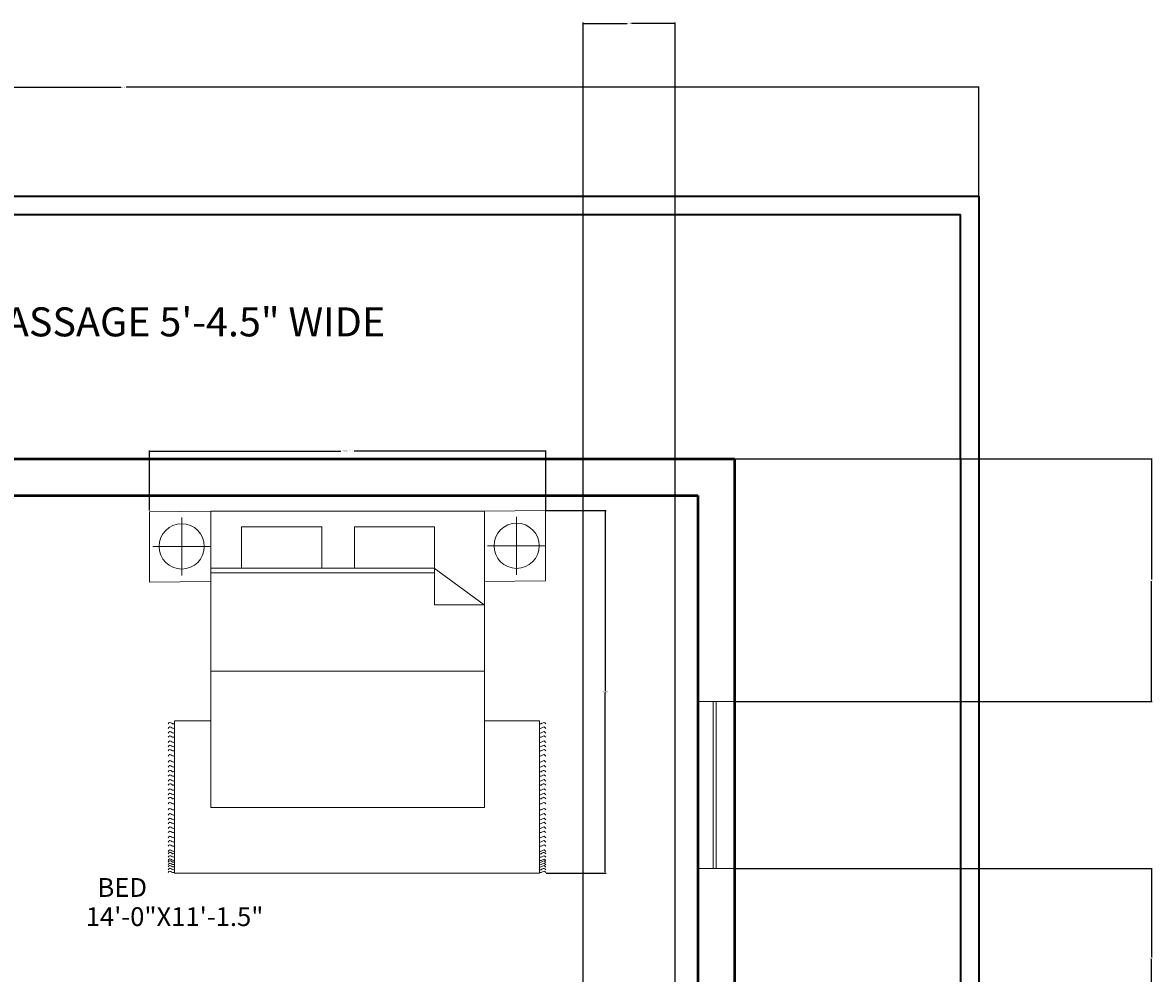
# Model space of a CAD drawing. Units: inches. Extents: x -44 to 461, y -6 to 860.
# Tile 7 of 7: x 184 to 461, y 626 to 860. Entities that reach past the tile are written whole.
import ezdxf

# ---------------------------------------------------------------- set-up
doc = ezdxf.new("R2010")
doc.units = ezdxf.units.IN
doc.header["$MEASUREMENT"] = 0
for name, color, linetype, lineweight in [('A-ANNO-DIMS', 2, 'Continuous', 18), ('A-AREA-IDEN', 7, 'Continuous', 18), ('C-PROP', 7, 'Continuous', 35), ('furniture', 30, 'Continuous', 18), ('walls', 8, 'Continuous', 50), ('windows', 171, 'Continuous', 18)]:
    doc.layers.add(name, color=color, linetype=linetype, lineweight=lineweight)
doc.styles.get("Standard").update_dxf_attribs({"font": 'arial.ttf'})
doc.dimstyles.get("Standard").update_dxf_attribs({"dimtxt": 0.18, "dimasz": 0.18, "dimexe": 0.18, "dimexo": 0.0625, "dimgap": 0.09, "dimtad": 0, "dimtih": 1, "dimtoh": 1, "dimdec": 4, "dimzin": 0, "dimdsep": 46, "dimtxsty": 'Standard', "dimcen": 0.09, "dimadec": 0, "dimazin": 0, "dimtfac": 1, "dimtdec": 4, "dimtofl": 0, "dimtmove": 0, "dimatfit": 3, "dimfxl": 1, "dimtolj": 1, "dimtzin": 0, "dimarcsym": 0})

# ---------------------------------------------------------------- blocks, each defined once
blk = doc.blocks.new('CARPET')
at = {"layer": 'furniture'}
for p, q in [((-51.53, -98.11), (-51.53, -55.12)), ((-51.53, -55.12), (-41.27, -55.12)), ((36, -55.12), (51.55, -55.12)), ((51.55, -55.12), (51.55, -98.11)), ((51.55, -98.11), (-51.53, -98.11))]:
    blk.add_line(p, q, dxfattribs=at)
for points, knots in [([(-53.37, -55.99), (-53.22, -55.8), (-52.9, -55.41), (-52.34, -55.8), (-51.89, -56.08), (-51.65, -55.91), (-51.53, -55.83)], [0, 0, 0, 0, 0.653278, 1.290138, 1.740457, 2.114451, 2.114451, 2.114451, 2.114451]), ([(-53.37, -57.26), (-53.22, -57.07), (-52.9, -56.67), (-52.34, -57.07), (-51.89, -57.35), (-51.65, -57.17), (-51.53, -57.1)], [0, 0, 0, 0, 0.653278, 1.290138, 1.740457, 2.114451, 2.114451, 2.114451, 2.114451]), ([(53.37, -55.99), (53.22, -55.8), (52.9, -55.41), (52.34, -55.8), (51.89, -56.08), (51.65, -55.91), (51.53, -55.83)], [0, 0, 0, 0, 0.653278, 1.290138, 1.740457, 2.114451, 2.114451, 2.114451, 2.114451]), ([(53.37, -57.26), (53.22, -57.07), (52.9, -56.67), (52.34, -57.07), (51.89, -57.35), (51.65, -57.17), (51.53, -57.1)], [0, 0, 0, 0, 0.653278, 1.290138, 1.740457, 2.114451, 2.114451, 2.114451, 2.114451]), ([(-53.37, -58.59), (-53.22, -58.4), (-52.9, -58.01), (-52.34, -58.4), (-51.89, -58.68), (-51.65, -58.5), (-51.53, -58.43)], [0, 0, 0, 0, 0.653278, 1.290138, 1.740457, 2.114451, 2.114451, 2.114451, 2.114451]), ([(-53.37, -59.78), (-53.22, -59.58), (-52.9, -59.19), (-52.34, -59.58), (-51.89, -59.86), (-51.65, -59.69), (-51.53, -59.61)], [0, 0, 0, 0, 0.653278, 1.290138, 1.740457, 2.114451, 2.114451, 2.114451, 2.114451]), ([(53.37, -58.59), (53.22, -58.4), (52.9, -58.01), (52.34, -58.4), (51.89, -58.68), (51.65, -58.5), (51.53, -58.43)], [0, 0, 0, 0, 0.653278, 1.290138, 1.740457, 2.114451, 2.114451, 2.114451, 2.114451]), ([(53.37, -59.78), (53.22, -59.58), (52.9, -59.19), (52.34, -59.58), (51.89, -59.86), (51.65, -59.69), (51.53, -59.61)], [0, 0, 0, 0, 0.653278, 1.290138, 1.740457, 2.114451, 2.114451, 2.114451, 2.114451]), ([(-53.37, -61.22), (-53.22, -61.02), (-52.9, -60.63), (-52.34, -61.02), (-51.89, -61.3), (-51.65, -61.13), (-51.53, -61.05)], [0, 0, 0, 0, 0.653278, 1.290138, 1.740457, 2.114451, 2.114451, 2.114451, 2.114451]), ([(-53.37, -62.44), (-53.22, -62.25), (-52.9, -61.86), (-52.34, -62.25), (-51.89, -62.53), (-51.65, -62.36), (-51.53, -62.28)], [0, 0, 0, 0, 0.653278, 1.290138, 1.740457, 2.114451, 2.114451, 2.114451, 2.114451]), ([(-53.37, -63.63), (-53.22, -63.43), (-52.9, -63.04), (-52.34, -63.43), (-51.89, -63.72), (-51.65, -63.54), (-51.53, -63.46)], [0, 0, 0, 0, 0.653278, 1.290138, 1.740457, 2.114451, 2.114451, 2.114451, 2.114451]), ([(53.37, -61.22), (53.22, -61.02), (52.9, -60.63), (52.34, -61.02), (51.89, -61.3), (51.65, -61.13), (51.53, -61.05)], [0, 0, 0, 0, 0.653278, 1.290138, 1.740457, 2.114451, 2.114451, 2.114451, 2.114451]), ([(53.37, -62.44), (53.22, -62.25), (52.9, -61.86), (52.34, -62.25), (51.89, -62.53), (51.65, -62.36), (51.53, -62.28)], [0, 0, 0, 0, 0.653278, 1.290138, 1.740457, 2.114451, 2.114451, 2.114451, 2.114451]), ([(53.37, -63.63), (53.22, -63.43), (52.9, -63.04), (52.34, -63.43), (51.89, -63.72), (51.65, -63.54), (51.53, -63.46)], [0, 0, 0, 0, 0.653278, 1.290138, 1.740457, 2.114451, 2.114451, 2.114451, 2.114451]), ([(-53.37, -65.07), (-53.22, -64.87), (-52.9, -64.48), (-52.34, -64.87), (-51.89, -65.15), (-51.65, -64.98), (-51.53, -64.9)], [0, 0, 0, 0, 0.653278, 1.290138, 1.740457, 2.114451, 2.114451, 2.114451, 2.114451]), ([(-53.37, -66.76), (-53.22, -66.56), (-52.9, -66.17), (-52.34, -66.56), (-51.89, -66.84), (-51.65, -66.67), (-51.53, -66.59)], [0, 0, 0, 0, 0.653278, 1.290138, 1.740457, 2.114451, 2.114451, 2.114451, 2.114451]), ([(53.37, -65.07), (53.22, -64.87), (52.9, -64.48), (52.34, -64.87), (51.89, -65.15), (51.65, -64.98), (51.53, -64.9)], [0, 0, 0, 0, 0.653278, 1.290138, 1.740457, 2.114451, 2.114451, 2.114451, 2.114451]), ([(53.37, -66.76), (53.22, -66.56), (52.9, -66.17), (52.34, -66.56), (51.89, -66.84), (51.65, -66.67), (51.53, -66.59)], [0, 0, 0, 0, 0.653278, 1.290138, 1.740457, 2.114451, 2.114451, 2.114451, 2.114451]), ([(-53.37, -68.2), (-53.22, -68), (-52.9, -67.61), (-52.34, -68), (-51.89, -68.28), (-51.65, -68.11), (-51.53, -68.03)], [0, 0, 0, 0, 0.653278, 1.290138, 1.740457, 2.114451, 2.114451, 2.114451, 2.114451]), ([(-53.37, -69.53), (-53.22, -69.33), (-52.9, -68.94), (-52.34, -69.33), (-51.89, -69.61), (-51.65, -69.44), (-51.53, -69.36)], [0, 0, 0, 0, 0.653278, 1.290138, 1.740457, 2.114451, 2.114451, 2.114451, 2.114451]), ([(53.37, -68.2), (53.22, -68), (52.9, -67.61), (52.34, -68), (51.89, -68.28), (51.65, -68.11), (51.53, -68.03)], [0, 0, 0, 0, 0.653278, 1.290138, 1.740457, 2.114451, 2.114451, 2.114451, 2.114451]), ([(53.37, -69.53), (53.22, -69.33), (52.9, -68.94), (52.34, -69.33), (51.89, -69.61), (51.65, -69.44), (51.53, -69.36)], [0, 0, 0, 0, 0.653278, 1.290138, 1.740457, 2.114451, 2.114451, 2.114451, 2.114451]), ([(-53.37, -70.79), (-53.22, -70.6), (-52.9, -70.21), (-52.34, -70.6), (-51.89, -70.88), (-51.65, -70.7), (-51.53, -70.63)], [0, 0, 0, 0, 0.653278, 1.290138, 1.740457, 2.114451, 2.114451, 2.114451, 2.114451]), ([(-53.37, -72.12), (-53.22, -71.93), (-52.9, -71.54), (-52.34, -71.93), (-51.89, -72.21), (-51.65, -72.04), (-51.53, -71.96)], [0, 0, 0, 0, 0.653278, 1.290138, 1.740457, 2.114451, 2.114451, 2.114451, 2.114451]), ([(-53.37, -73.31), (-53.22, -73.11), (-52.9, -72.72), (-52.34, -73.11), (-51.89, -73.4), (-51.65, -73.22), (-51.53, -73.14)], [0, 0, 0, 0, 0.653278, 1.290138, 1.740457, 2.114451, 2.114451, 2.114451, 2.114451]), ([(53.37, -70.79), (53.22, -70.6), (52.9, -70.21), (52.34, -70.6), (51.89, -70.88), (51.65, -70.7), (51.53, -70.63)], [0, 0, 0, 0, 0.653278, 1.290138, 1.740457, 2.114451, 2.114451, 2.114451, 2.114451]), ([(53.37, -72.12), (53.22, -71.93), (52.9, -71.54), (52.34, -71.93), (51.89, -72.21), (51.65, -72.04), (51.53, -71.96)], [0, 0, 0, 0, 0.653278, 1.290138, 1.740457, 2.114451, 2.114451, 2.114451, 2.114451]), ([(53.37, -73.31), (53.22, -73.11), (52.9, -72.72), (52.34, -73.11), (51.89, -73.4), (51.65, -73.22), (51.53, -73.14)], [0, 0, 0, 0, 0.653278, 1.290138, 1.740457, 2.114451, 2.114451, 2.114451, 2.114451]), ([(-53.37, -74.75), (-53.22, -74.55), (-52.9, -74.16), (-52.34, -74.55), (-51.89, -74.83), (-51.65, -74.66), (-51.53, -74.58)], [0, 0, 0, 0, 0.653278, 1.290138, 1.740457, 2.114451, 2.114451, 2.114451, 2.114451]), ([(-53.37, -75.98), (-53.22, -75.78), (-52.9, -75.39), (-52.34, -75.78), (-51.89, -76.06), (-51.65, -75.89), (-51.53, -75.81)], [0, 0, 0, 0, 0.653278, 1.290138, 1.740457, 2.114451, 2.114451, 2.114451, 2.114451]), ([(53.37, -74.75), (53.22, -74.55), (52.9, -74.16), (52.34, -74.55), (51.89, -74.83), (51.65, -74.66), (51.53, -74.58)], [0, 0, 0, 0, 0.653278, 1.290138, 1.740457, 2.114451, 2.114451, 2.114451, 2.114451]), ([(53.37, -75.98), (53.22, -75.78), (52.9, -75.39), (52.34, -75.78), (51.89, -76.06), (51.65, -75.89), (51.53, -75.81)], [0, 0, 0, 0, 0.653278, 1.290138, 1.740457, 2.114451, 2.114451, 2.114451, 2.114451]), ([(-53.37, -77.16), (-53.22, -76.96), (-52.9, -76.57), (-52.34, -76.96), (-51.89, -77.25), (-51.65, -77.07), (-51.53, -76.99)], [0, 0, 0, 0, 0.653278, 1.290138, 1.740457, 2.114451, 2.114451, 2.114451, 2.114451]), ([(-53.37, -78.6), (-53.22, -78.4), (-52.9, -78.01), (-52.34, -78.4), (-51.89, -78.68), (-51.65, -78.51), (-51.53, -78.43)], [0, 0, 0, 0, 0.653278, 1.290138, 1.740457, 2.114451, 2.114451, 2.114451, 2.114451]), ([(-53.37, -80.29), (-53.22, -80.09), (-52.9, -79.7), (-52.34, -80.09), (-51.89, -80.37), (-51.65, -80.2), (-51.53, -80.12)], [0, 0, 0, 0, 0.653278, 1.290138, 1.740457, 2.114451, 2.114451, 2.114451, 2.114451]), ([(53.37, -77.16), (53.22, -76.96), (52.9, -76.57), (52.34, -76.96), (51.89, -77.25), (51.65, -77.07), (51.53, -76.99)], [0, 0, 0, 0, 0.653278, 1.290138, 1.740457, 2.114451, 2.114451, 2.114451, 2.114451]), ([(53.37, -78.6), (53.22, -78.4), (52.9, -78.01), (52.34, -78.4), (51.89, -78.68), (51.65, -78.51), (51.53, -78.43)], [0, 0, 0, 0, 0.653278, 1.290138, 1.740457, 2.114451, 2.114451, 2.114451, 2.114451]), ([(53.37, -80.29), (53.22, -80.09), (52.9, -79.7), (52.34, -80.09), (51.89, -80.37), (51.65, -80.2), (51.53, -80.12)], [0, 0, 0, 0, 0.653278, 1.290138, 1.740457, 2.114451, 2.114451, 2.114451, 2.114451]), ([(-53.37, -81.73), (-53.22, -81.53), (-52.9, -81.14), (-52.34, -81.53), (-51.89, -81.81), (-51.65, -81.64), (-51.53, -81.56)], [0, 0, 0, 0, 0.653278, 1.290138, 1.740457, 2.114451, 2.114451, 2.114451, 2.114451]), ([(-53.37, -83.06), (-53.22, -82.86), (-52.9, -82.47), (-52.34, -82.86), (-51.89, -83.14), (-51.65, -82.97), (-51.53, -82.89)], [0, 0, 0, 0, 0.653278, 1.290138, 1.740457, 2.114451, 2.114451, 2.114451, 2.114451]), ([(53.37, -81.73), (53.22, -81.53), (52.9, -81.14), (52.34, -81.53), (51.89, -81.81), (51.65, -81.64), (51.53, -81.56)], [0, 0, 0, 0, 0.653278, 1.290138, 1.740457, 2.114451, 2.114451, 2.114451, 2.114451]), ([(53.37, -83.06), (53.22, -82.86), (52.9, -82.47), (52.34, -82.86), (51.89, -83.14), (51.65, -82.97), (51.53, -82.89)], [0, 0, 0, 0, 0.653278, 1.290138, 1.740457, 2.114451, 2.114451, 2.114451, 2.114451]), ([(-53.37, -84.18), (-53.22, -83.99), (-52.9, -83.6), (-52.34, -83.99), (-51.89, -84.27), (-51.65, -84.09), (-51.53, -84.02)], [0, 0, 0, 0, 0.653278, 1.290138, 1.740457, 2.114451, 2.114451, 2.114451, 2.114451]), ([(-53.37, -85.51), (-53.22, -85.32), (-52.9, -84.93), (-52.34, -85.32), (-51.89, -85.6), (-51.65, -85.42), (-51.53, -85.35)], [0, 0, 0, 0, 0.653278, 1.290138, 1.740457, 2.114451, 2.114451, 2.114451, 2.114451]), ([(-53.37, -86.7), (-53.22, -86.5), (-52.9, -86.11), (-52.34, -86.5), (-51.89, -86.78), (-51.65, -86.61), (-51.53, -86.53)], [0, 0, 0, 0, 0.653278, 1.290138, 1.740457, 2.114451, 2.114451, 2.114451, 2.114451]), ([(53.37, -84.18), (53.22, -83.99), (52.9, -83.6), (52.34, -83.99), (51.89, -84.27), (51.65, -84.09), (51.53, -84.02)], [0, 0, 0, 0, 0.653278, 1.290138, 1.740457, 2.114451, 2.114451, 2.114451, 2.114451]), ([(53.37, -85.51), (53.22, -85.32), (52.9, -84.93), (52.34, -85.32), (51.89, -85.6), (51.65, -85.42), (51.53, -85.35)], [0, 0, 0, 0, 0.653278, 1.290138, 1.740457, 2.114451, 2.114451, 2.114451, 2.114451]), ([(53.37, -86.7), (53.22, -86.5), (52.9, -86.11), (52.34, -86.5), (51.89, -86.78), (51.65, -86.61), (51.53, -86.53)], [0, 0, 0, 0, 0.653278, 1.290138, 1.740457, 2.114451, 2.114451, 2.114451, 2.114451]), ([(-53.37, -88.14), (-53.22, -87.94), (-52.9, -87.55), (-52.34, -87.94), (-51.89, -88.22), (-51.65, -88.05), (-51.53, -87.97)], [0, 0, 0, 0, 0.653278, 1.290138, 1.740457, 2.114451, 2.114451, 2.114451, 2.114451]), ([(-53.37, -89.36), (-53.22, -89.17), (-52.9, -88.78), (-52.34, -89.17), (-51.89, -89.45), (-51.65, -89.28), (-51.53, -89.2)], [0, 0, 0, 0, 0.653278, 1.290138, 1.740457, 2.114451, 2.114451, 2.114451, 2.114451]), ([(53.37, -88.14), (53.22, -87.94), (52.9, -87.55), (52.34, -87.94), (51.89, -88.22), (51.65, -88.05), (51.53, -87.97)], [0, 0, 0, 0, 0.653278, 1.290138, 1.740457, 2.114451, 2.114451, 2.114451, 2.114451]), ([(53.37, -89.36), (53.22, -89.17), (52.9, -88.78), (52.34, -89.17), (51.89, -89.45), (51.65, -89.28), (51.53, -89.2)], [0, 0, 0, 0, 0.653278, 1.290138, 1.740457, 2.114451, 2.114451, 2.114451, 2.114451]), ([(-53.37, -90.55), (-53.22, -90.35), (-52.9, -89.96), (-52.34, -90.35), (-51.89, -90.64), (-51.65, -90.46), (-51.53, -90.38)], [0, 0, 0, 0, 0.653278, 1.290138, 1.740457, 2.114451, 2.114451, 2.114451, 2.114451]), ([(-53.37, -91.99), (-53.22, -91.79), (-52.9, -91.4), (-52.34, -91.79), (-51.89, -92.07), (-51.65, -91.9), (-51.53, -91.82)], [0, 0, 0, 0, 0.653278, 1.290138, 1.740457, 2.114451, 2.114451, 2.114451, 2.114451]), ([(-53.37, -92.69), (-53.22, -92.48), (-52.9, -92.08), (-52.35, -92.49), (-51.89, -92.77), (-51.65, -92.6), (-51.53, -92.52)], [0, 0, 0, 0, 0.663904, 1.307406, 1.757725, 2.131719, 2.131719, 2.131719, 2.131719]), ([(53.37, -90.55), (53.22, -90.35), (52.9, -89.96), (52.34, -90.35), (51.9, -90.63), (51.66, -90.47), (51.55, -90.4)], [0, 0, 0, 0, 0.653278, 1.290138, 1.740457, 2.0926, 2.0926, 2.0926, 2.0926]), ([(53.37, -91.99), (53.22, -91.79), (52.9, -91.4), (52.34, -91.79), (51.9, -92.07), (51.66, -91.91), (51.55, -91.83)], [0, 0, 0, 0, 0.653278, 1.290138, 1.740457, 2.0926, 2.0926, 2.0926, 2.0926]), ([(53.37, -92.69), (53.22, -92.49), (52.9, -92.09), (52.34, -92.49), (51.9, -92.77), (51.66, -92.61), (51.55, -92.53)], [0, 0, 0, 0, 0.656792, 1.295826, 1.746145, 2.098292, 2.098292, 2.098292, 2.098292]), ([(-53.37, -93.61), (-53.22, -93.42), (-52.9, -93.03), (-52.34, -93.42), (-51.89, -93.7), (-51.65, -93.52), (-51.53, -93.45)], [0, 0, 0, 0, 0.653278, 1.290138, 1.740457, 2.114451, 2.114451, 2.114451, 2.114451]), ([(-53.37, -94.55), (-53.22, -94.35), (-52.9, -93.96), (-52.34, -94.35), (-51.89, -94.63), (-51.65, -94.46), (-51.53, -94.38)], [0, 0, 0, 0, 0.653278, 1.290138, 1.740457, 2.114451, 2.114451, 2.114451, 2.114451]), ([(-53.37, -95.05), (-53.22, -94.85), (-52.9, -94.46), (-52.34, -94.85), (-51.89, -95.14), (-51.65, -94.96), (-51.53, -94.88)], [0, 0, 0, 0, 0.653278, 1.290138, 1.740457, 2.114451, 2.114451, 2.114451, 2.114451]), ([(-53.37, -95.73), (-53.22, -95.54), (-52.9, -95.15), (-52.34, -95.54), (-51.89, -95.82), (-51.65, -95.65), (-51.53, -95.57)], [0, 0, 0, 0, 0.653278, 1.290138, 1.740457, 2.114451, 2.114451, 2.114451, 2.114451]), ([(53.37, -95.78), (53.22, -95.58), (52.9, -95.19), (52.34, -95.58), (51.89, -95.86), (51.65, -95.69), (51.53, -95.61)], [0, 0, 0, 0, 0.653278, 1.290138, 1.740457, 2.114451, 2.114451, 2.114451, 2.114451]), ([(53.37, -93.66), (53.22, -93.46), (52.9, -93.07), (52.34, -93.46), (51.9, -93.74), (51.66, -93.58), (51.55, -93.5)], [0, 0, 0, 0, 0.653278, 1.290138, 1.740457, 2.0926, 2.0926, 2.0926, 2.0926]), ([(53.37, -94.59), (53.22, -94.4), (52.9, -94.01), (52.34, -94.4), (51.9, -94.68), (51.66, -94.51), (51.55, -94.44)], [0, 0, 0, 0, 0.653278, 1.290138, 1.740457, 2.0926, 2.0926, 2.0926, 2.0926]), ([(53.37, -95.1), (53.22, -94.9), (52.9, -94.51), (52.34, -94.9), (51.9, -95.18), (51.66, -95.02), (51.55, -94.94)], [0, 0, 0, 0, 0.653278, 1.290138, 1.740457, 2.0926, 2.0926, 2.0926, 2.0926]), ([(-53.37, -96.38), (-53.22, -96.18), (-52.9, -95.79), (-52.34, -96.18), (-51.89, -96.47), (-51.65, -96.29), (-51.53, -96.21)], [0, 0, 0, 0, 0.653278, 1.290138, 1.740457, 2.114451, 2.114451, 2.114451, 2.114451]), ([(-53.37, -97.17), (-53.22, -96.98), (-52.9, -96.59), (-52.34, -96.98), (-51.89, -97.26), (-51.65, -97.08), (-51.53, -97.01)], [0, 0, 0, 0, 0.653278, 1.290138, 1.740457, 2.114451, 2.114451, 2.114451, 2.114451]), ([(-53.37, -97.99), (-53.22, -97.79), (-52.9, -97.4), (-52.34, -97.79), (-51.89, -98.08), (-51.65, -97.9), (-51.53, -97.82)], [0, 0, 0, 0, 0.653278, 1.290138, 1.740457, 2.114451, 2.114451, 2.114451, 2.114451]), ([(53.37, -96.43), (53.22, -96.23), (52.9, -95.84), (52.34, -96.23), (51.89, -96.51), (51.65, -96.34), (51.53, -96.26)], [0, 0, 0, 0, 0.653278, 1.290138, 1.740457, 2.114451, 2.114451, 2.114451, 2.114451]), ([(53.37, -97.22), (53.22, -97.02), (52.9, -96.63), (52.34, -97.02), (51.89, -97.3), (51.65, -97.13), (51.53, -97.05)], [0, 0, 0, 0, 0.653278, 1.290138, 1.740457, 2.114451, 2.114451, 2.114451, 2.114451]), ([(53.37, -97.99), (53.22, -97.79), (52.9, -97.4), (52.34, -97.79), (51.89, -98.08), (51.65, -97.9), (51.53, -97.82)], [0, 0, 0, 0, 0.653278, 1.290138, 1.740457, 2.114451, 2.114451, 2.114451, 2.114451])]:
    blk.add_open_spline(points, degree=3, knots=knots, dxfattribs=at)
blk = doc.blocks.new('A$C58D270C6')
at = {"layer": 'furniture'}
for p, q in [((9.09, 124.13), (9.09, 108.87)), ((1.46, 116.5), (16.73, 116.5)), ((14.97, 94.84), (24.62, 107.92)), ((24.62, 94.93), (24.62, 107.92)), ((42.08, 108), (42.08, 36)), ((14.97, 94.93), (24.62, 94.93)), ((14.97, 94.84), (14.97, 36)), ((16.22, 94.93), (16.22, 36)), ((9.25, 36), (9.25, 20.74)), ((1.62, 28.37), (16.88, 28.37))]:
    blk.add_line(p, q, dxfattribs=at)
for points in [[(18.5, 108), (18.34, 124.13), (-0.16, 124.13), (0, 108)], [(0, 108), (77.91, 108), (77.91, 36), (0, 36)], [(4.09, 94.93), (14.97, 94.93), (14.97, 73.83), (4.09, 73.83)], [(4.09, 65.23), (14.97, 65.23), (14.97, 44.13), (4.09, 44.13)], [(18.65, 19.87), (18.5, 36), (0, 36), (0.16, 19.87)]]:
    blk.add_lwpolyline(points, close=True, dxfattribs=at)
for centre in [(9.09, 116.5), (9.25, 28.37)]:
    blk.add_circle(centre, 5.95, dxfattribs=at)
at = {"layer": 'furniture', "xscale": 0.9312884925094044, "yscale": 0.9312884925094044, "zscale": 0.9312884925094044, "rotation": 90}
blk.add_blockref('CARPET', (3.79, 74.47), dxfattribs=at)
blk = doc.blocks.new('*D18')
at = {"layer": 'A-ANNO-DIMS', "color": 0, "lineweight": -2, "transparency": 16777216}
for p, q in [((-1.55, 817.11), (-1.55, 843.94)), ((-1.37, 843.76), (207.84, 843.76)), ((418.27, 843.76), (209.05, 843.76)), ((418.45, 817.11), (418.45, 843.94))]:
    blk.add_line(p, q, dxfattribs=at)
at = {"layer": 'A-ANNO-DIMS', "color": 0, "transparency": 16777216}
for points in [[(-1.37, 843.79), (-1.37, 843.73), (-1.55, 843.76)], [(418.27, 843.79), (418.27, 843.73), (418.45, 843.76)]]:
    blk.add_solid(points, dxfattribs=at)
at = {"layer": 'Defpoints', "color": 0, "transparency": 16777216}
for p in [(418.45, 843.76), (-1.55, 817.05), (418.45, 817.05)]:
    blk.add_point(p, dxfattribs=at)
at = {"layer": 'A-ANNO-DIMS', "color": 0, "transparency": 16777216, "insert": (208.45, 843.76), "char_height": 0.18, "attachment_point": 5}
blk.add_mtext('\\A1;420.0000', dxfattribs=at)
blk = doc.blocks.new('WIN-41IN-FRAME')
for p, q in [((0, 40.98), (9, 40.98)), ((0, 40.98), (0, 0)), ((3.73, 40.98), (3.73, 0)), ((4.5, 0), (4.5, 40.98)), ((9, 40.98), (9, 0)), ((9, 0), (0, 0))]:
    blk.add_line(p, q)
blk = doc.blocks.new('*D38')
at = {"layer": 'A-ANNO-DIMS', "color": 0, "lineweight": -2, "transparency": 16777216}
for p, q in [((214.77, 739.94), (214.77, 754.66)), ((214.95, 754.48), (261.81, 754.48)), ((311.93, 754.48), (265.07, 754.48)), ((312.11, 739.94), (312.11, 754.66))]:
    blk.add_line(p, q, dxfattribs=at)
at = {"layer": 'A-ANNO-DIMS', "color": 0, "transparency": 16777216}
for points in [[(214.95, 754.51), (214.95, 754.45), (214.77, 754.48)], [(311.93, 754.51), (311.93, 754.45), (312.11, 754.48)]]:
    blk.add_solid(points, dxfattribs=at)
at = {"layer": 'Defpoints', "color": 0, "transparency": 16777216}
for p in [(312.11, 754.48), (214.77, 739.88), (312.11, 739.88)]:
    blk.add_point(p, dxfattribs=at)
at = {"layer": 'A-ANNO-DIMS', "color": 0, "transparency": 16777216, "insert": (263.44, 754.48), "char_height": 0.18, "attachment_point": 5}
blk.add_mtext('\\A1;BED GROUP 97.3411 TYP.', dxfattribs=at)
blk = doc.blocks.new('*D39')
at = {"layer": 'A-ANNO-DIMS', "color": 0, "lineweight": -2, "transparency": 16777216}
for p, q in [((312.17, 739.88), (326.89, 739.88)), ((326.71, 739.7), (326.71, 695.59)), ((326.71, 651.12), (326.71, 695.23)), ((312.17, 650.94), (326.89, 650.94))]:
    blk.add_line(p, q, dxfattribs=at)
at = {"layer": 'A-ANNO-DIMS', "color": 0, "transparency": 16777216}
for points in [[(326.68, 739.7), (326.74, 739.7), (326.71, 739.88)], [(326.68, 651.12), (326.74, 651.12), (326.71, 650.94)]]:
    blk.add_solid(points, dxfattribs=at)
at = {"layer": 'Defpoints', "color": 0, "transparency": 16777216}
for p in [(312.11, 739.88), (312.11, 650.94), (326.71, 650.94)]:
    blk.add_point(p, dxfattribs=at)
at = {"layer": 'A-ANNO-DIMS', "color": 0, "transparency": 16777216, "insert": (326.71, 695.41), "char_height": 0.18, "attachment_point": 5}
blk.add_mtext('\\A1;88.9451 TYP.', dxfattribs=at)
blk = doc.blocks.new('*D53')
at = {"layer": 'A-ANNO-DIMS', "color": 0, "lineweight": -2, "transparency": 16777216}
for p, q in [((321.29, 454.3), (321.29, 859.63)), ((321.47, 859.45), (332.05, 859.45)), ((343.69, 859.45), (333.11, 859.45)), ((343.87, 454.3), (343.87, 859.63))]:
    blk.add_line(p, q, dxfattribs=at)
at = {"layer": 'A-ANNO-DIMS', "color": 0, "transparency": 16777216}
for points in [[(321.47, 859.48), (321.47, 859.42), (321.29, 859.45)], [(343.69, 859.48), (343.69, 859.42), (343.87, 859.45)]]:
    blk.add_solid(points, dxfattribs=at)
at = {"layer": 'Defpoints', "color": 0, "transparency": 16777216}
for p in [(343.87, 859.45), (321.29, 454.23), (343.87, 454.23)]:
    blk.add_point(p, dxfattribs=at)
at = {"layer": 'A-ANNO-DIMS', "color": 0, "transparency": 16777216, "insert": (332.58, 859.45), "char_height": 0.18, "attachment_point": 5}
blk.add_mtext('\\A1;22.5824', dxfattribs=at)
blk = doc.blocks.new('*D59')
at = {"layer": 'A-ANNO-DIMS', "color": 0, "lineweight": -2, "transparency": 16777216}
for p, q in [((358.51, 752.55), (461.03, 752.55)), ((460.85, 752.37), (460.85, 722.96)), ((460.85, 693.19), (460.85, 722.6)), ((358.51, 693.01), (461.03, 693.01))]:
    blk.add_line(p, q, dxfattribs=at)
at = {"layer": 'A-ANNO-DIMS', "color": 0, "transparency": 16777216}
for points in [[(460.82, 752.37), (460.88, 752.37), (460.85, 752.55)], [(460.82, 693.19), (460.88, 693.19), (460.85, 693.01)]]:
    blk.add_solid(points, dxfattribs=at)
at = {"layer": 'Defpoints', "color": 0, "transparency": 16777216}
for p in [(358.45, 752.55), (358.45, 693.01), (460.85, 693.01)]:
    blk.add_point(p, dxfattribs=at)
at = {"layer": 'A-ANNO-DIMS', "color": 0, "transparency": 16777216, "insert": (460.85, 722.78), "char_height": 0.18, "attachment_point": 5}
blk.add_mtext('\\A1;59.5423', dxfattribs=at)
blk = doc.blocks.new('*D60')
at = {"layer": 'A-ANNO-DIMS', "color": 0, "lineweight": -2, "transparency": 16777216}
for p, q in [((358.51, 652.02), (461.03, 652.02)), ((460.85, 651.84), (460.85, 630.26)), ((460.85, 608.32), (460.85, 629.9)), ((358.51, 608.14), (461.03, 608.14))]:
    blk.add_line(p, q, dxfattribs=at)
at = {"layer": 'A-ANNO-DIMS', "color": 0, "transparency": 16777216}
for points in [[(460.82, 651.84), (460.88, 651.84), (460.85, 652.02)], [(460.82, 608.32), (460.88, 608.32), (460.85, 608.14)]]:
    blk.add_solid(points, dxfattribs=at)
at = {"layer": 'Defpoints', "color": 0, "transparency": 16777216}
for p in [(358.45, 652.02), (358.45, 608.14), (460.85, 608.14)]:
    blk.add_point(p, dxfattribs=at)
at = {"layer": 'A-ANNO-DIMS', "color": 0, "transparency": 16777216, "insert": (460.85, 630.08), "char_height": 0.18, "attachment_point": 5}
blk.add_mtext('\\A1;43.8805', dxfattribs=at)

msp = doc.modelspace()

# ---------------------------------------------------------------- linework, layer by layer
at = {"layer": 'C-PROP'}
for p, q in [((-1.55432, 817.0501), (418.44568, 817.0501)), ((418.44568, 817.0501), (418.44568, 37.0501)), ((2.94568, 812.5501), (413.94568, 812.5501)), ((413.94568, 752.5501), (413.94568, 812.5501)), ((413.94568, 752.5501), (413.94568, 262.0501))]:
    msp.add_line(p, q, dxfattribs=at)
at = {"layer": 'walls'}
for p, q in [((-1.55432, 752.5501), (358.44568, 752.5501)), ((358.44568, 752.5501), (358.44568, 262.0501)), ((155.94568, 743.5501), (349.44568, 743.5501)), ((349.44568, 743.5501), (349.44568, 610.0501))]:
    msp.add_line(p, q, dxfattribs=at)

# ---------------------------------------------------------------- block references
at = {"layer": 'furniture', "xscale": 0.9331788672991836, "yscale": 0.9331788672991836, "zscale": 0.9331788672991836, "rotation": 269.9999999999999}
msp.add_blockref('A$C58D270C6', (196.22691, 739.73538), dxfattribs=at)
at = {"layer": 'windows'}
msp.add_blockref('WIN-41IN-FRAME', (349.446, 652.023), dxfattribs=at)

# ---------------------------------------------------------------- texts
at = {"layer": 'A-AREA-IDEN'}
for s, height, p in [('PASSAGE 5\'-4.5" WIDE', 7.1129656, (173.13701, 782.63673)), ('BED', 4.610309, (202.0242, 645.09766)), ('14\'-0"X11\'-1.5"', 4.6103088, (199.13964, 637.93311))]:
    msp.add_text(s, height=height, dxfattribs=at).set_placement(p)

# ---------------------------------------------------------------- dimensions: what is measured, and where the dimension line sits
at = {"layer": 'A-ANNO-DIMS'}
for base, p1, p2, override, picture, middle in [((343.87134, 859.4501), (321.28892, 454.23298), (343.87134, 454.23298), {"dimdec": 4, "dimlfac": 1, "dimrnd": 0, "dimzin": 0, "dimdsep": 46, "dimlunit": 2}, '*D53', (332.58013, 859.4501)), ((418.44568, 843.76223), (-1.55432, 817.0501), (418.44568, 817.0501), {"dimclrd": 0, "dimclre": 0, "dimclrt": 0}, '*D18', (208.44568, 843.76223))]:
    dim = msp.add_linear_dim(base=base, p1=p1, p2=p2, dimstyle='Standard', override=override, dxfattribs=at)
    dim.commit()
    dim.dimension.update_dxf_attribs({"geometry": picture, "text_midpoint": middle})
dim = msp.add_linear_dim(base=(312.10923, 754.48168), p1=(214.76814, 739.88052), p2=(312.10923, 739.88052), text='BED GROUP <> TYP.', dimstyle='Standard', override={"dimdec": 4, "dimlfac": 1, "dimrnd": 0, "dimzin": 0, "dimdsep": 46, "dimlunit": 2}, dxfattribs=at)
dim.commit()
dim.dimension.update_dxf_attribs({"geometry": '*D38', "text_midpoint": (263.43868, 754.48168)})
for base, p1, p2, picture, middle in [((460.84569, 693.00783), (358.44569, 752.5501), (358.44569, 693.00783), '*D59', (460.84569, 722.77897)), ((460.84569, 608.14262), (358.44569, 652.02311), (358.44569, 608.14262), '*D60', (460.84569, 630.08287))]:
    dim = msp.add_linear_dim(base=base, p1=p1, p2=p2, angle=90, dimstyle='Standard', override={"dimdec": 4, "dimlfac": 1, "dimrnd": 0, "dimzin": 0, "dimdsep": 46, "dimlunit": 2}, dxfattribs=at)
    dim.commit()
    dim.dimension.update_dxf_attribs({"geometry": picture, "text_midpoint": middle})
dim = msp.add_linear_dim(base=(326.71039, 650.93539), p1=(312.10923, 739.88052), p2=(312.10923, 650.93539), angle=270, text='<> TYP.', dimstyle='Standard', override={"dimdec": 4, "dimlfac": 1, "dimrnd": 0, "dimzin": 0, "dimdsep": 46, "dimlunit": 2}, dxfattribs=at)
dim.commit()
dim.dimension.update_dxf_attribs({"geometry": '*D39', "text_midpoint": (326.71039, 695.40796)})

doc.saveas('drawing.dxf')
